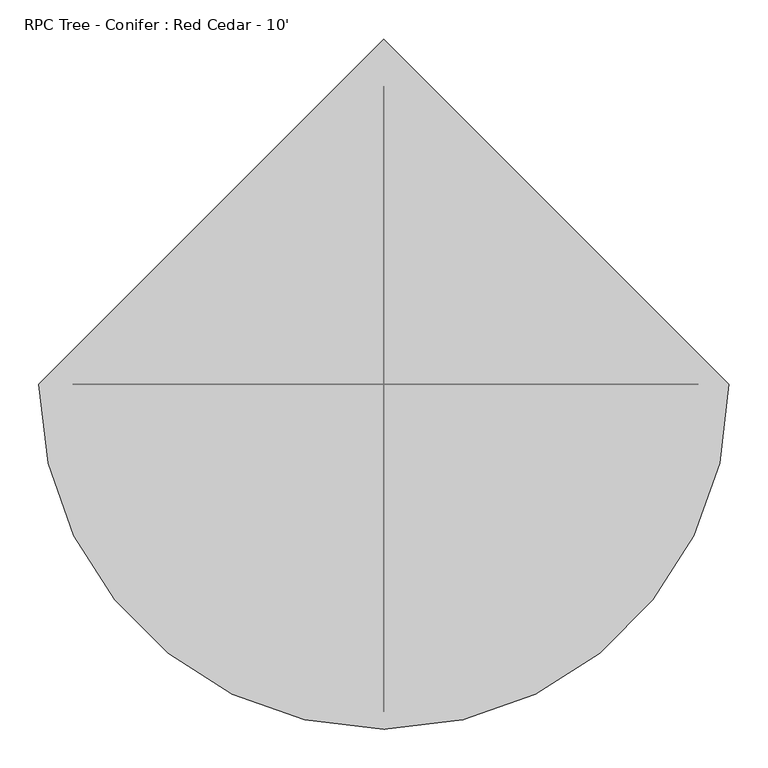
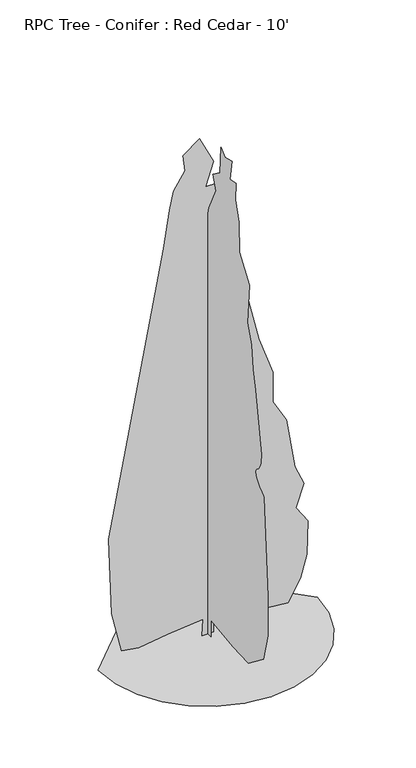
"""IFC4 building model written with IfcOpenShell, lengths in millimetres: geographic element geometry, RPC Tree - Conifer : Red Cedar - 10'."""

from ifc_helpers import new_model, si_unit, origin, place, context, project, spatial, triangles, source, transform, mapped, element, save


def rpc_tree_conifer_red_cedar_10_c53c74b4(model_context):
    return source(origin(), model_context, "Body", "Tessellation", [
        triangles([(-23.2585186, 1e-06, 2.1e-06), (-19.6360221, -3.2e-06, 68.825818), (-163.403271, 3.8e-06, 55.5663894), (-279.7066552, 9.9e-06, 38.4378564), (-349.2744292, 1.23e-05, 50.7136968), (-389.1211613, 3.8e-06, 220.9662), (-399.9883032, -1.49e-05, 543.3619283), (-338.4072873, -3.7e-05, 869.3776754), (-179.0221032, -9.39e-05, 1706.1538525), (-153.6651662, -0.0001043, 1861.9207981), (-139.1755347, -0.0001094, 1937.9835972), (-92.0841594, -0.0001158, 2010.4371689), (-99.3289752, -0.0001194, 2075.6363869), (-34.1256514, -0.0001252, 2126.3626511), (23.8328589, -0.0001209, 2010.4371689), (-8.7687661, -0.0001136, 1912.6293308), (34.7001689, -0.0001155, 1912.6293308), (207.1184442, -7.97e-05, 1186.0695368), (262.912059, -7.26e-05, 1025.1410603), (262.912059, -6.5e-05, 898.3572292), (317.2477504, -6.18e-05, 804.174824), (353.4726831, -5.06e-05, 590.4522225), (389.6958718, -4.73e-05, 507.1369592), (357.0944824, -4.02e-05, 412.9545539), (404.1865571, -3.8e-05, 340.5064324), (400.5630137, -2.94e-05, 199.2319343), (375.206967, -2.27e-05, 105.0498833), (324.493093, -1.53e-05, 18.1121235), (239.5580339, -1.21e-05, 28.0987891), (121.6379333, -6.8e-06, 25.356937), (23.8328589, -4.7e-06, 61.5810068), (23.8328589, -1e-06, 0.0), (0.196672, 20.5351814, 6.44e-05), (0.1966706, 27.7799949, 50.713874), (0.1966755, 82.7498636, 17.6619693), (0.1966773, 183.5428665, 47.0913798), (0.1966776, 161.8091277, 76.0706338), (0.1966835, 295.8377382, 76.0706338), (0.1966866, 353.7969729, 90.5602608), (0.1966907, 364.6641149, 173.8757059), (0.1966943, 382.7765631, 326.0174912), (0.1966957, 357.4187359, 383.9749638), (0.1967, 361.0423156, 478.1573327), (0.1967016, 335.6844884, 539.7383486), (0.1967043, 324.8173465, 702.747076), (0.196705, 277.7270522, 764.3281282), (0.1967117, 212.5224748, 1072.2331713), (0.1967154, 140.0745169, 1318.5571621), (0.1967172, 89.3609972, 1499.6783741), (0.1967169, 64.0040647, 1517.7890419), (0.1967201, 42.2696219, 1611.9715199), (0.1967233, -8.4441277, 1825.7029507), (0.1967255, -59.1579488, 1927.1201614), (0.1967251, -37.423506, 1985.0829025), (0.1967247, -84.5148813, 2021.30075), (0.1967292, -91.7596971, 2133.599128), (0.1967269, -120.7389511, 2108.2448616), (0.1967253, -167.8301446, 2119.1084427), (0.1967221, -156.9630209, 2035.7914352), (0.1967207, -196.810298, 2043.0456436), (0.1967177, -193.1867364, 1970.5922173), (0.196717, -218.5445636, 1890.902314), (0.1967113, -222.1663447, 1764.1131054), (0.1967078, -293.3254279, 1666.4565662), (0.1967011, -276.5019998, 1496.0547581), (0.1966965, -305.4816081, 1419.9848373), (0.1966956, -316.34875, 1322.1788887), (0.1966913, -334.4612346, 1242.4872414), (0.1966826, -374.3079666, 992.5396345), (0.196682, -374.2119696, 980.1310169), (0.1966815, -373.5469666, 967.7846048), (0.1966811, -371.7405361, 955.5661646), (0.1966807, -368.223636, 943.5379744), (0.1966804, -362.4255887, 931.7623123), (0.1966803, -353.7774247, 920.3031281), (0.1966804, -341.7065772, 909.2243711), (0.1966801, -334.3616404, 896.380097), (0.1966793, -337.9052104, 880.7408627), (0.1966781, -348.7776572, 864.0454428), (0.1966767, -363.4248373, 848.0345741), (0.1966755, -378.2906814, 834.4435432), (0.1966746, -389.8174487, 825.0147583), (0.1966781, -394.4491427, 821.4836512), (0.1966629, -421.3982609, 412.9545539), (0.1966595, -421.3982609, 246.3240272), (0.1966557, -388.7968715, 126.7843306), (0.1966568, -283.7473424, 47.0913798), (0.1966618, -175.0747969, 50.7136968), (0.1966694, -22.9337019, 72.4481351), (0.1966701, -22.9337019, 6.18e-05), (-443.1865748, 0.0, 8.26e-05), (-431.4642162, -101.5939896, 7.6e-05), (-398.0822785, -194.8918286, 6.9e-05), (-345.7095305, -277.2203063, 6.18e-05), (-277.0236431, -345.9062119, 5.47e-05), (-194.6951654, -398.2789598, 4.8e-05), (-101.3973174, -431.6608975, 4.19e-05), (0.1966906, -443.3832561, 3.68e-05), (101.7906618, -431.6608975, 3.3e-05), (195.0884917, -398.2789598, 9.31e-05), (277.4169694, -345.9062119, 9.27e-05), (346.1046736, -277.2203063, 9.38e-05), (398.4756412, -194.8918286, 3.42e-05), (431.8575788, -101.5939896, 3.83e-05), (443.5799375, 3.88e-05, 4.38e-05), (0.1966127, 443.3832561, 8.96e-05)], [[13, 14, 15], [12, 13, 15], [12, 15, 16], [11, 12, 16], [32, 1, 2], [31, 32, 2], [10, 11, 16], [16, 17, 18], [10, 16, 18], [9, 10, 18], [8, 9, 18], [8, 18, 19], [8, 19, 20], [7, 8, 20], [7, 20, 21], [7, 21, 22], [6, 7, 22], [6, 22, 23], [6, 23, 24], [5, 6, 24], [4, 5, 24], [3, 4, 24], [2, 3, 24], [31, 2, 24], [30, 31, 24], [29, 30, 24], [29, 24, 25], [29, 25, 26], [29, 26, 27], [29, 27, 28], [55, 56, 57], [35, 36, 37], [57, 58, 59], [55, 57, 59], [59, 60, 61], [89, 90, 33], [89, 33, 34], [53, 54, 55], [55, 59, 61], [53, 55, 61], [53, 61, 62], [52, 53, 62], [52, 62, 63], [51, 52, 63], [51, 63, 64], [51, 64, 65], [50, 51, 65], [38, 39, 40], [34, 35, 37], [50, 65, 66], [50, 66, 67], [49, 50, 67], [48, 49, 67], [48, 67, 68], [47, 48, 68], [47, 68, 69], [46, 47, 69], [46, 69, 70], [46, 70, 71], [46, 71, 72], [46, 72, 73], [46, 73, 74], [46, 74, 75], [46, 75, 76], [46, 76, 77], [46, 77, 78], [46, 78, 79], [46, 79, 80], [37, 38, 40], [37, 40, 41], [37, 41, 42], [46, 80, 81], [82, 83, 84], [34, 37, 42], [89, 34, 42], [89, 42, 43], [89, 43, 44], [45, 46, 81], [44, 45, 81], [89, 44, 81], [88, 89, 81], [88, 81, 82], [88, 82, 84], [88, 84, 85], [88, 85, 86], [88, 86, 87], [105, 106, 91], [104, 105, 91], [104, 91, 92], [103, 104, 92], [103, 92, 93], [103, 93, 94], [102, 103, 94], [101, 102, 94], [101, 94, 95], [101, 95, 96], [101, 96, 97], [101, 97, 98], [101, 98, 99], [101, 99, 100]], closed=False),
    ])


if __name__ == "__main__":
    model = new_model("IFC4")
    model_context = context("Model", 3, world=origin())
    ifc_project = project(units=[si_unit("LENGTHUNIT", "METRE", prefix="MILLI")], contexts=[model_context])
    site = spatial("IfcSite", under=ifc_project)
    building = spatial("IfcBuilding", under=site)
    placement = place(None, origin())
    rpc_tree_conifer_red_cedar_10_shape = rpc_tree_conifer_red_cedar_10_c53c74b4(model_context)
    element("IfcGeographicElement", 1, ObjectType="RPC Tree - Conifer : Red Cedar - 10'", at=placement, inside=building, context=model_context, shape_type="MappedRepresentation", body=[
        mapped(rpc_tree_conifer_red_cedar_10_shape, transform((0.0, 0.0, 0.0), x_axis=(1.0, 0.0, 0.0), y_axis=(0.0, 1.0, 0.0), z_axis=(0.0, 0.0, 1.0))),
    ])
    save(model, "model.ifc")

# Revit data of these elements
# Type "RPC Tree - Conifer : Red Cedar - 10'"
#   built-in parameter 1005198 = "{2, 15},{39, RPC-16-FXGH-CPG0-PPQ3-C000-ST1L-LVER-AU},{1, 0},{1, 0},{2, 35},{1, 8},{5, Color},{1, 0},{1, 0},{3, 0.8},{3, 0.8},{3, 0.8},{1, 8},{7, BBoxMin},{1, 0},{1, 0},{1, 0},{1, 0},{1, 0},{1, 8},{7, BBoxMax},{1, 0},{1, 0},{1, 0},{1, 0},{1, 0},{2, 11},{9, RPCTypeId},{1, 0},{1, 0},{39, RPC-16-FXGH-CPG0-PPQ3-C000-ST1L-LVER-AU},{1, 6},{14, RPCPlantHeight},{1, 0},{1, 0},{2, 10},{2, 11},{7, keyword},{1, 0},{1, 0},{99, :Geometry:RPC:Red Cedar:red cedar:western:cupressacae:thuja plicata:north america:evergreen:conifer},{2, 11},{8, category},{1, 0},{1, 0},{16, :Trees [General]},{2, 11},{12, LocalizedUID},{1, 0},{1, 0},{9, Red Cedar},{2, 14},{6, Height},{1, 0},{1, 0},{2, 10},{1, 2},{16, Cast Reflections},{1, 0},{1, 0},{1, 0},{1, 2},{12, Cast Shadows},{1, 0},{1, 0},{1, 1},{1, 2},{9, Lock View},{1, 0},{1, 0},{1, 0},{1, 4},{5, ViewC},{1, 0},{1, 0},{1, 0},{2, 11},{20, AdvancedUIDefinition},{1, 0},{1, 0},{0, },{2, 11},{10, AssetLibID},{1, 0},{1, 0},{36, 4D3F6E72-3F99-4203-98E9-AF80B3C7A7A4},{2, 11},{10, BaseSchema},{1, 0},{1, 0},{9, RPCSchema},{2, 11},{12, ExchangeGUID},{1, 0},{1, 0},{0, },{1, 2},{6, Hidden},{1, 0},{1, 0},{1, 0},{1, 4},{11, RPCCategory},{1, 0},{1, 0},{1, 0},{2, 11},{8, RPCImage},{1, 0},{1, 0},{0, },{1, 4},{13, SchemaVersion},{1, 0},{1, 0},{1, 4},{2, 11},{12, UIDefinition},{1, 0},{1, 0},{0, },{2, 11},{6, UIName},{1, 0},{1, 0},{39, RPC-16-FXGH-CPG0-PPQ3-C000-ST1L-LVER-AU},{2, 11},{11, VersionGUID},{1, 0},{1, 0},{9, RPCSchema},{2, 11},{9, assettype},{1, 0},{1, 0},{11, RPCGeometry},{2, 11},{11, description},{1, 0},{1, 0},{0, },{2, 11},{9, localname},{1, 0},{1, 0},{3, RPC},{2, 11},{9, localtype},{1, 0},{1, 0},{3, RPC},{1, 4},{8, revision},{1, 0},{1, 0},{1, 1},{2, 11},{9, thumbnail},{1, 0},{1, 0},{0, },{1, 4},{7, version},{1, 0},{1, 0},{1, 1},{1, 2},{20, RPC_Cast Reflections},{1, 0},{1, 0},{1, 1},{1, 2},{16, RPC_Cast Shadows},{1, 0},{1, 0},{1, 1},{1, 2},{13, RPC_Lock View},{1, 0},{1, 0},{1, 0},{1, 4},{9, RPC_ViewC},{1, 0},{1, 0},{1, 0},{21, assetlibrary_base.fbx},{1, 5},"
#   built-in parameter 1005195 = "RPC-16-FXGH-CPG0-PPQ3-C000-ST1L-LVER-AU"
#   Type Comments = "Red Cedar"
#   Assembly Code = "G2050500"
#   Height = 7' - 0"
#   Description = (empty or 0)
#   Default Elevation = 0
